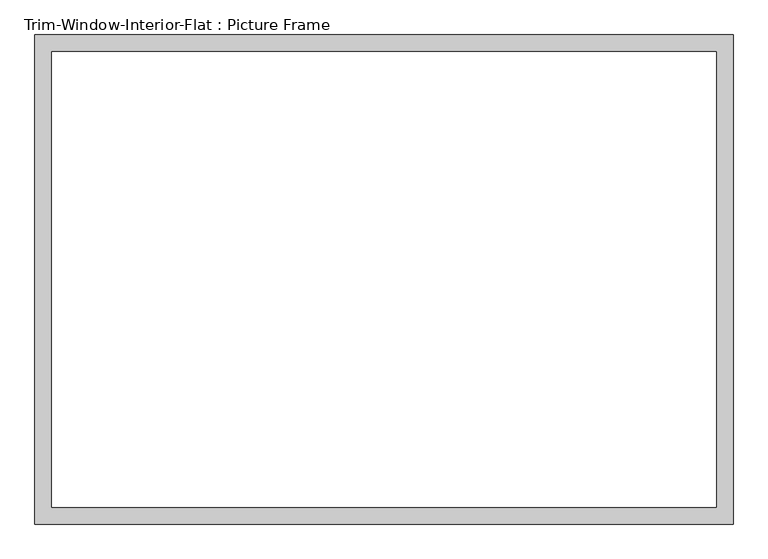
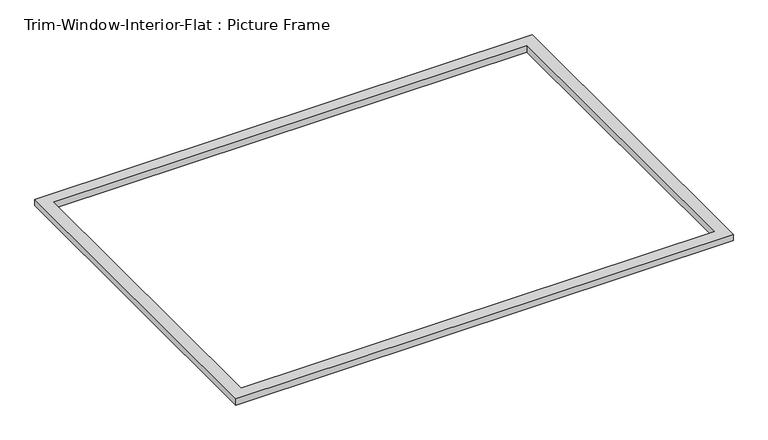
"""IFC4 building model written with IfcOpenShell, lengths in millimetres: proxy geometry, Trim-Window-Interior-Flat : Picture Frame."""

from ifc_helpers import new_model, si_unit, origin, origin_with_axes, place, context, project, spatial, polyline, outline, extrude, source, transform, mapped, element, save


def trim_window_interior_flat_picture_frame_9ca7b173(model_context):
    return source(origin(), model_context, "Body", "SweptSolid", [
        extrude(outline(polyline([(1187.45, 44.45), (1187.45, -1619.25), (-1187.45, -1619.25), (-1187.45, 44.45), (1187.45, 44.45)]), holes=[polyline([(1130.3, -12.7), (-1130.3, -12.7), (-1130.3, -1562.1), (1130.3, -1562.1), (1130.3, -12.7)])]), origin_with_axes(), (0.0, 0.0, 1.0), 31.75),
    ])


if __name__ == "__main__":
    model = new_model("IFC4")
    model_context = context("Model", 3, world=origin())
    ifc_project = project(units=[si_unit("LENGTHUNIT", "METRE", prefix="MILLI")], contexts=[model_context])
    site = spatial("IfcSite", under=ifc_project)
    building = spatial("IfcBuilding", under=site)
    placement = place(None, origin())
    trim_window_interior_flat_picture_frame_shape = trim_window_interior_flat_picture_frame_9ca7b173(model_context)
    element("IfcBuildingElementProxy", 1, Name="Trim-Window-Interior-Flat : Picture Frame", ObjectType="Trim-Window-Interior-Flat : Picture Frame", at=placement, inside=building, context=model_context, shape_type="MappedRepresentation", body=[
        mapped(trim_window_interior_flat_picture_frame_shape, transform((0.0, 0.0, 0.0), x_axis=(1.0, 0.0, 0.0), y_axis=(0.0, 1.0, 0.0), z_axis=(0.0, 0.0, 1.0))),
    ])
    save(model, "model.ifc")

# Revit data of these elements
# Type "Trim-Window-Interior-Flat : Picture Frame"
#   Trim Thickness_Picture Frame = 0' - 1 1/4"
#   Trim Width = 0' - 2 1/4"
#   Trim Thickness_with Sill = 0' - 0 3/4"
#   Sill Thickness = 0' - 1 1/4"
#   Opening Width [instance default] = 2' - 0"
#   Opening Height [instance default] = 3' - 0"
#   Default Elevation = 4' - 0"
#   Sill = no
#   Picture Frame = yes
#   Trim Material [instance default] = none
# Element 1 (IfcBuildingElementProxy, "Trim-Window-Interior-Flat : Picture Frame")
#   Opening Width = 7' - 6"
#   Opening Height = 5' - 2"
#   Trim Material = Wood - Stained
#   Materials on its faces: "Wood - Stained"
# Materials
#   "Wood - Stained": class "Wood", colour RGB 224 178 126, transparency 0, Cost = 0
